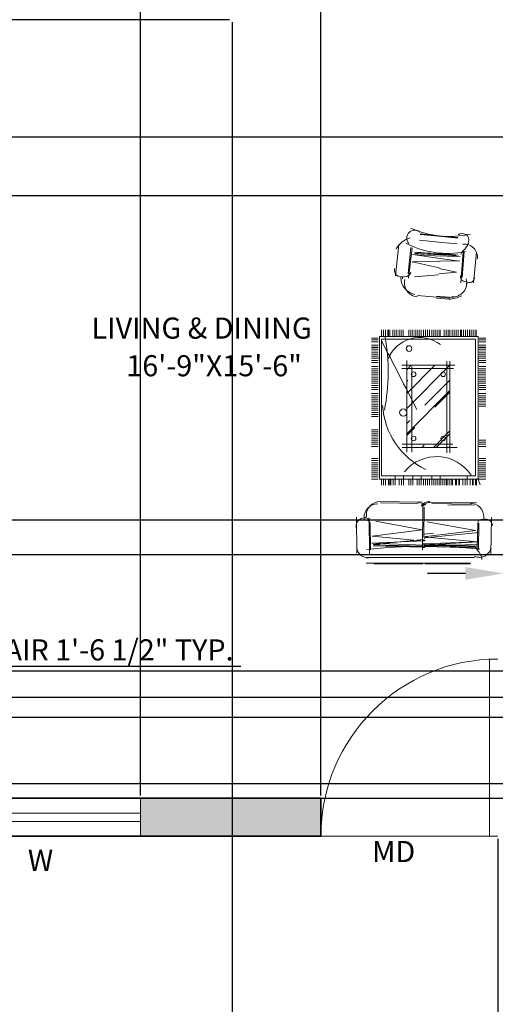
# Model space of a CAD drawing. Units: inches. Extents: x 2265 to 2807, y 1544 to 2401.
# Tile 7 of 9: x 2531 to 2643, y 1890 to 2124. Entities that reach past the tile are written whole.
import ezdxf

# ---------------------------------------------------------------- set-up
doc = ezdxf.new("R2010")
doc.units = ezdxf.units.IN
for name, color, linetype, lineweight in [('A-ANNO-DIMS', 2, 'Continuous', 18), ('A-ANNO-TEXT', 7, 'Continuous', 18), ('A-AREA-IDEN', 7, 'Continuous', 18), ('A-DOOR', 3, 'Continuous', 18), ('A-FURN-PATT', 161, 'Continuous', 13), ('A-GLAZ', 4, 'Continuous', 18), ('A-WALL', 7, 'Continuous', 35), ('A-WALL-PATT', 18, 'Continuous', 13), ('Furniture', 161, 'Continuous', 15)]:
    doc.layers.add(name, color=color, linetype=linetype, lineweight=lineweight)
doc.styles.add('ARIAL', font='times.ttf', dxfattribs={"height": 5})
doc.styles.get("Standard").update_dxf_attribs({"font": 'arial.ttf', "height": 5})
doc.dimstyles.new('ISO-25', dxfattribs={"dimtxt": 5, "dimasz": 9, "dimexe": 1.25, "dimexo": 0.625, "dimtad": 1, "dimlunit": 3, "dimtxsty": 'Standard', "dimcen": 2.5, "dimadec": 0, "dimazin": 0, "dimtfac": 1, "dimtmove": 0, "dimatfit": 3, "dimfxl": 1, "dimarcsym": 0})

# ---------------------------------------------------------------- blocks, each defined once
blk = doc.blocks.new('GLAZING-48IN')
for p, q in [((48, 9), (0, 9)), ((0, 5.5), (48, 5.5)), ((0, 5.5), (48, 5.5)), ((0, 3.5), (48, 3.5)), ((0, 0), (48, 0))]:
    blk.add_line(p, q)
blk = doc.blocks.new('DOOR-SWING-42IN')
for p, q in [((40, 41.95), (40, 0)), ((42, 0), (0, 0))]:
    blk.add_line(p, q)
blk.add_arc((42, 0), 42, 90, 180)
blk = doc.blocks.new('*D27')
at = {"layer": 'A-ANNO-DIMS', "color": 0, "lineweight": -2, "transparency": 16777216}
for p, q in [((2479.74, 1968.41), (2479.74, 1971.79)), ((2498.12, 1968.41), (2498.12, 1971.79)), ((2470.74, 1970.54), (2461.74, 1970.54)), ((2479.74, 1970.54), (2498.12, 1970.54)), ((2507.12, 1970.54), (2583.11, 1970.54))]:
    blk.add_line(p, q, dxfattribs=at)
at = {"layer": 'A-ANNO-DIMS', "color": 0, "lineweight": 100, "transparency": 16777216}
for points in [[(2470.74, 1972.04), (2470.74, 1969.04), (2479.74, 1970.54)], [(2507.12, 1972.04), (2507.12, 1969.04), (2498.12, 1970.54)]]:
    blk.add_solid(points, dxfattribs=at)
at = {"layer": 'Defpoints', "color": 0, "lineweight": 100, "transparency": 16777216}
for p in [(2498.12, 1970.54), (2479.74, 1967.79), (2498.12, 1967.79)]:
    blk.add_point(p, dxfattribs=at)
at = {"layer": 'A-ANNO-DIMS', "color": 0, "transparency": 16777216, "insert": (2549.62, 1973.75), "char_height": 5, "attachment_point": 5}
blk.add_mtext('CHAIR 1\'-6 1/2" TYP.', dxfattribs=at)
blk = doc.blocks.new('*D29')
at = {"layer": 'A-ANNO-DIMS', "color": 0, "lineweight": -2, "transparency": 16777216}
for p, q in [((2645.38, 1993.96), (2645.38, 1991.27)), ((2659.2, 1993.96), (2659.2, 1991.27)), ((2636.38, 1992.52), (2627.38, 1992.52)), ((2645.38, 1992.52), (2659.2, 1992.52)), ((2668.2, 1992.52), (2749.43, 1992.52))]:
    blk.add_line(p, q, dxfattribs=at)
at = {"layer": 'A-ANNO-DIMS', "color": 0, "lineweight": 100, "transparency": 16777216}
for points in [[(2636.38, 1994.02), (2636.38, 1991.02), (2645.38, 1992.52)], [(2668.2, 1994.02), (2668.2, 1991.02), (2659.2, 1992.52)]]:
    blk.add_solid(points, dxfattribs=at)
at = {"layer": 'Defpoints', "color": 0, "lineweight": 100, "transparency": 16777216}
for p in [(2645.38, 1994.59), (2659.2, 1994.59), (2659.2, 1992.52)]:
    blk.add_point(p, dxfattribs=at)
at = {"layer": 'A-ANNO-DIMS', "color": 0, "transparency": 16777216, "insert": (2713.31, 1995.65), "char_height": 5, "attachment_point": 5}
blk.add_mtext('END TABLE 1\'-2" TYP.', dxfattribs=at)
blk = doc.blocks.new('*D35')
at = {"layer": 'A-ANNO-DIMS', "color": 0, "lineweight": -2, "transparency": 16777216}
for p, q in [((2581.1, 2123.11), (2581.1, 1546.93)), ((2662.1, 2123.11), (2662.1, 1546.93)), ((2590.1, 1548.18), (2653.1, 1548.18))]:
    blk.add_line(p, q, dxfattribs=at)
at = {"layer": 'A-ANNO-DIMS', "color": 0, "lineweight": 100, "transparency": 16777216}
for points in [[(2590.1, 1549.68), (2590.1, 1546.68), (2581.1, 1548.18)], [(2653.1, 1549.68), (2653.1, 1546.68), (2662.1, 1548.18)]]:
    blk.add_solid(points, dxfattribs=at)
at = {"layer": 'Defpoints', "color": 0, "lineweight": 100, "transparency": 16777216}
for p in [(2581.1, 2123.73), (2662.1, 2123.73), (2662.1, 1548.18)]:
    blk.add_point(p, dxfattribs=at)
at = {"layer": 'A-ANNO-DIMS', "color": 0, "transparency": 16777216, "insert": (2621.6, 1551.36), "char_height": 5, "attachment_point": 5}
blk.add_mtext('6\'-9"', dxfattribs=at)
blk = doc.blocks.new('*D39')
at = {"layer": 'A-ANNO-DIMS', "color": 0, "lineweight": -2, "transparency": 16777216}
for p, q in [((2644.1, 1929.61), (2644.1, 1546.93)), ((2662.1, 1929.61), (2662.1, 1546.93)), ((2635.1, 1548.18), (2626.1, 1548.18)), ((2644.1, 1548.18), (2662.1, 1548.18)), ((2671.1, 1548.18), (2680.1, 1548.18))]:
    blk.add_line(p, q, dxfattribs=at)
at = {"layer": 'A-ANNO-DIMS', "color": 0, "lineweight": 100, "transparency": 16777216}
for points in [[(2635.1, 1549.68), (2635.1, 1546.68), (2644.1, 1548.18)], [(2671.1, 1549.68), (2671.1, 1546.68), (2662.1, 1548.18)]]:
    blk.add_solid(points, dxfattribs=at)
at = {"layer": 'Defpoints', "color": 0, "lineweight": 100, "transparency": 16777216}
for p in [(2644.1, 1930.23), (2662.1, 1930.23), (2662.1, 1548.18)]:
    blk.add_point(p, dxfattribs=at)
at = {"layer": 'A-ANNO-DIMS', "color": 0, "transparency": 16777216, "insert": (2653.1, 1551.36), "char_height": 5, "attachment_point": 5}
blk.add_mtext('1\'-6"', dxfattribs=at)
blk = doc.blocks.new('*D41')
at = {"layer": 'A-ANNO-DIMS', "color": 0, "lineweight": -2, "transparency": 16777216}
for p, q in [((2392.73, 2005.23), (2804.46, 2005.23)), ((2803.21, 1996.23), (2803.21, 1972.23)), ((2392.73, 1963.23), (2804.46, 1963.23))]:
    blk.add_line(p, q, dxfattribs=at)
at = {"layer": 'A-ANNO-DIMS', "color": 0, "lineweight": 100, "transparency": 16777216}
for points in [[(2801.71, 1996.23), (2804.71, 1996.23), (2803.21, 2005.23)], [(2801.71, 1972.23), (2804.71, 1972.23), (2803.21, 1963.23)]]:
    blk.add_solid(points, dxfattribs=at)
at = {"layer": 'Defpoints', "color": 0, "lineweight": 100, "transparency": 16777216}
for p in [(2392.1, 2005.23), (2392.1, 1963.23), (2803.21, 1963.23)]:
    blk.add_point(p, dxfattribs=at)
at = {"layer": 'A-ANNO-DIMS', "color": 0, "transparency": 16777216, "insert": (2800.03, 1984.23), "char_height": 5, "attachment_point": 5, "rotation": 90}
blk.add_mtext('3\'-6"', dxfattribs=at)
blk = doc.blocks.new('*D42')
at = {"layer": 'A-ANNO-DIMS', "color": 0, "lineweight": -2, "transparency": 16777216}
for p, q in [((2464.73, 1963.23), (2804.46, 1963.23)), ((2803.21, 1954.23), (2803.21, 1948.23)), ((2464.73, 1939.23), (2804.46, 1939.23))]:
    blk.add_line(p, q, dxfattribs=at)
at = {"layer": 'A-ANNO-DIMS', "color": 0, "lineweight": 100, "transparency": 16777216}
for points in [[(2801.71, 1954.23), (2804.71, 1954.23), (2803.21, 1963.23)], [(2801.71, 1948.23), (2804.71, 1948.23), (2803.21, 1939.23)]]:
    blk.add_solid(points, dxfattribs=at)
at = {"layer": 'Defpoints', "color": 0, "lineweight": 100, "transparency": 16777216}
for p in [(2464.1, 1963.23), (2464.1, 1939.23), (2803.21, 1939.23)]:
    blk.add_point(p, dxfattribs=at)
at = {"layer": 'A-ANNO-DIMS', "color": 0, "transparency": 16777216, "insert": (2800.03, 1951.23), "char_height": 5, "attachment_point": 5, "rotation": 90}
blk.add_mtext('2\'-0"', dxfattribs=at)
blk = doc.blocks.new('*D46')
at = {"layer": 'A-ANNO-DIMS', "color": 0, "lineweight": -2, "transparency": 16777216}
for p, q in [((2803.21, 2104.95), (2803.21, 2128.02)), ((2381.23, 2095.95), (2804.46, 2095.95)), ((2803.21, 2082.06), (2803.21, 2095.95)), ((2381.23, 2082.06), (2804.46, 2082.06)), ((2803.21, 2073.06), (2803.21, 2064.06))]:
    blk.add_line(p, q, dxfattribs=at)
at = {"layer": 'A-ANNO-DIMS', "color": 0, "lineweight": 100, "transparency": 16777216}
for points in [[(2801.71, 2104.95), (2804.71, 2104.95), (2803.21, 2095.95)], [(2801.71, 2073.06), (2804.71, 2073.06), (2803.21, 2082.06)]]:
    blk.add_solid(points, dxfattribs=at)
at = {"layer": 'Defpoints', "color": 0, "lineweight": 100, "transparency": 16777216}
for p in [(2380.61, 2095.95), (2803.21, 2095.95), (2380.61, 2082.06)]:
    blk.add_point(p, dxfattribs=at)
at = {"layer": 'A-ANNO-DIMS', "color": 0, "transparency": 16777216, "insert": (2800.07, 2120.99), "char_height": 5, "attachment_point": 5, "rotation": 90}
blk.add_mtext('1\'-2"', dxfattribs=at)
blk = doc.blocks.new('*D52')
at = {"layer": 'A-ANNO-DIMS', "color": 0, "lineweight": -2, "transparency": 16777216}
for p, q in [((2559.35, 1939.86), (2559.35, 2297.59)), ((2568.35, 2296.34), (2593.1, 2296.34)), ((2602.1, 1939.86), (2602.1, 2297.59))]:
    blk.add_line(p, q, dxfattribs=at)
at = {"layer": 'A-ANNO-DIMS', "color": 0, "lineweight": 100, "transparency": 16777216}
for points in [[(2568.35, 2297.84), (2568.35, 2294.84), (2559.35, 2296.34)], [(2593.1, 2297.84), (2593.1, 2294.84), (2602.1, 2296.34)]]:
    blk.add_solid(points, dxfattribs=at)
at = {"layer": 'Defpoints', "color": 0, "lineweight": 100, "transparency": 16777216}
for p in [(2602.1, 2296.34), (2559.35, 1939.23), (2602.1, 1939.23)]:
    blk.add_point(p, dxfattribs=at)
at = {"layer": 'A-ANNO-DIMS', "color": 0, "transparency": 16777216, "insert": (2580.73, 2299.52), "char_height": 5, "attachment_point": 5}
blk.add_mtext('3\'-7"', dxfattribs=at)
blk = doc.blocks.new('*D60')
at = {"layer": 'A-ANNO-DIMS', "color": 0, "lineweight": -2, "transparency": 16777216}
for p, q in [((2275.29, 2142.73), (2275.29, 2151.73)), ((2580.48, 2133.73), (2274.04, 2133.73)), ((2275.29, 2133.73), (2275.29, 2123.73)), ((2580.48, 2123.73), (2274.04, 2123.73)), ((2275.29, 2114.73), (2275.29, 2087.31))]:
    blk.add_line(p, q, dxfattribs=at)
at = {"layer": 'A-ANNO-DIMS', "color": 0, "lineweight": 100, "transparency": 16777216}
for points in [[(2273.79, 2142.73), (2276.79, 2142.73), (2275.29, 2133.73)], [(2273.79, 2114.73), (2276.79, 2114.73), (2275.29, 2123.73)]]:
    blk.add_solid(points, dxfattribs=at)
at = {"layer": 'Defpoints', "color": 0, "lineweight": 100, "transparency": 16777216}
for p in [(2581.1, 2133.73), (2275.29, 2123.73), (2581.1, 2123.73)]:
    blk.add_point(p, dxfattribs=at)
at = {"layer": 'A-ANNO-DIMS', "color": 0, "transparency": 16777216, "insert": (2272.11, 2096.52), "char_height": 5, "attachment_point": 5, "rotation": 90}
blk.add_mtext('0\'-10"', dxfattribs=at)
blk = doc.blocks.new('*D61')
at = {"layer": 'A-ANNO-DIMS', "color": 0, "lineweight": -2, "transparency": 16777216}
for p, q in [((2803.21, 1967.45), (2803.21, 1976.45)), ((2444.67, 1958.45), (2804.46, 1958.45)), ((2803.21, 1958.45), (2803.21, 1942.7)), ((2444.67, 1942.7), (2804.46, 1942.7)), ((2803.21, 1933.7), (2803.21, 1898.98))]:
    blk.add_line(p, q, dxfattribs=at)
at = {"layer": 'A-ANNO-DIMS', "color": 0, "lineweight": 100, "transparency": 16777216}
for points in [[(2801.71, 1967.45), (2804.71, 1967.45), (2803.21, 1958.45)], [(2801.71, 1933.7), (2804.71, 1933.7), (2803.21, 1942.7)]]:
    blk.add_solid(points, dxfattribs=at)
at = {"layer": 'Defpoints', "color": 0, "lineweight": 100, "transparency": 16777216}
for p in [(2444.05, 1958.45), (2444.05, 1942.7), (2803.21, 1942.7)]:
    blk.add_point(p, dxfattribs=at)
at = {"layer": 'A-ANNO-DIMS', "color": 0, "transparency": 16777216, "insert": (2800, 1911.84), "char_height": 5, "attachment_point": 5, "rotation": 90}
blk.add_mtext('1\'-3 1/2"', dxfattribs=at)
blk = doc.blocks.new('*D64')
at = {"layer": 'A-ANNO-DIMS', "color": 0, "lineweight": -2, "transparency": 16777216}
for p, q in [((2521.03, 1996.97), (2804.46, 1996.97)), ((2803.21, 1978.41), (2803.21, 1987.97)), ((2521.03, 1969.41), (2804.46, 1969.41))]:
    blk.add_line(p, q, dxfattribs=at)
at = {"layer": 'A-ANNO-DIMS', "color": 0, "lineweight": 100, "transparency": 16777216}
for points in [[(2801.71, 1987.97), (2804.71, 1987.97), (2803.21, 1996.97)], [(2801.71, 1978.41), (2804.71, 1978.41), (2803.21, 1969.41)]]:
    blk.add_solid(points, dxfattribs=at)
at = {"layer": 'Defpoints', "color": 0, "lineweight": 100, "transparency": 16777216}
for p in [(2520.4, 1996.97), (2803.21, 1996.97), (2520.4, 1969.41)]:
    blk.add_point(p, dxfattribs=at)
at = {"layer": 'A-ANNO-DIMS', "color": 0, "transparency": 16777216, "insert": (2800, 1983.19), "char_height": 5, "attachment_point": 5, "rotation": 90}
blk.add_mtext('2\'-3 1/2"', dxfattribs=at)

msp = doc.modelspace()

# ---------------------------------------------------------------- hatches: boundary and pattern name
at = {"layer": 'A-FURN-PATT'}
h = msp.add_hatch(dxfattribs=at)
h.set_pattern_fill('AR-RROOF', color=256, scale=0.266265, angle=585, style=0)
h.set_pattern_definition([(225, (3863.236, 2357.7255), (-5.7387, -15.3032), [101.44684, -13.52625, 33.8156, -6.76312]), (225, (3859.267, 2348.974), (11.14264, -1.57814), [20.28937, -2.23183, 40.57874, -5.07234]), (225, (3864.91, 2351.2695), (-21.663592, -28.071807), [54.10498, -9.46837, 27.05249, -6.76312])])
h.paths.add_polyline_path([(2622.465, 2022.355), (2632.719, 2022.355), (2632.719, 2041.841), (2622.465, 2041.841)])
at = {"layer": 'A-WALL-PATT'}
h = msp.add_hatch(color=256, dxfattribs=at)
h.dxf.hatch_style = 1
h.paths.add_polyline_path([(2602.101, 1939.233), (2559.351, 1939.233), (2559.351, 1930.233), (2602.101, 1930.233)])

# ---------------------------------------------------------------- linework, layer by layer
at = {"layer": 'A-GLAZ'}
msp.add_line((2559.351, 1930.233), (2559.351, 1939.233), dxfattribs=at)
at = {"layer": 'A-WALL'}
for p, q in [((2602.101, 1939.233), (2468.601, 1939.233)), ((2602.101, 1939.233), (2602.101, 1930.233)), ((2602.101, 1930.233), (2368.101, 1930.233))]:
    msp.add_line(p, q, dxfattribs=at)
at = {"layer": 'Furniture'}
for p, q in [((2625.638, 2072.819), (2630.883, 2072.324)), ((2625.652, 2072.969), (2630.897, 2072.474)), ((2630.883, 2072.324), (2634.557, 2071.977)), ((2630.897, 2072.474), (2634.571, 2072.127)), ((2619.772, 2063.047), (2620.583, 2070.456)), ((2622.77, 2063.613), (2623.459, 2069.781)), ((2622.875, 2062.461), (2623.723, 2069.661)), ((2625.511, 2071.467), (2630.756, 2070.972)), ((2630.756, 2070.972), (2634.43, 2070.625)), ((2630.397, 2067.172), (2623.848, 2068.074)), ((2623.848, 2068.074), (2630.449, 2067.722)), ((2630.453, 2067.769), (2635.095, 2067.522)), ((2635.281, 2061.372), (2635.805, 2068.741)), ((2635.608, 2062.621), (2636.086, 2068.809)), ((2639.033, 2068.684), (2638.324, 2061.402)), ((2630.325, 2066.416), (2623.791, 2066.374)), ((2623.791, 2066.374), (2630.186, 2064.946)), ((2635.021, 2066.564), (2630.336, 2066.534)), ((2634.941, 2066.496), (2630.392, 2067.123)), ((2621.534, 2062.871), (2621.467, 2062.288)), ((2622.041, 2062.787), (2621.758, 2062.82)), ((2630.029, 2063.284), (2624.329, 2062.775)), ((2634.294, 2063.879), (2630.05, 2063.5)), ((2630.173, 2064.799), (2634.294, 2063.879)), ((2621.985, 2062.173), (2621.942, 2061.587)), ((2621.985, 2062.173), (2621.942, 2061.587)), ((2636.169, 2061.674), (2636.454, 2061.653)), ((2636.683, 2061.661), (2636.64, 2061.076)), ((2629.531, 2058.002), (2625.026, 2058.35)), ((2632.71, 2057.777), (2629.532, 2058.022)), ((2633.538, 2057.935), (2629.553, 2058.243)), ((2632.498, 2057.501), (2629.505, 2057.731)), ((2616.007, 2048.698), (2639.384, 2048.698)), ((2616.007, 2014.891), (2616.007, 2048.698)), ((2616.486, 2048.705), (2616.486, 2050.258)), ((2616.979, 2048.705), (2616.979, 2050.258)), ((2617.472, 2048.705), (2617.472, 2050.258)), ((2617.965, 2048.705), (2617.965, 2050.258)), ((2618.153, 2048.705), (2618.153, 2050.258)), ((2618.459, 2048.705), (2618.459, 2050.258)), ((2619.159, 2048.705), (2619.159, 2050.258)), ((2619.652, 2048.705), (2619.652, 2050.258)), ((2620.145, 2048.705), (2620.145, 2050.258)), ((2620.639, 2048.705), (2620.639, 2050.258)), ((2621.132, 2048.705), (2621.132, 2050.258)), ((2621.625, 2048.705), (2621.625, 2050.258)), ((2622.955, 2048.705), (2622.955, 2050.258)), ((2623.449, 2048.705), (2623.449, 2050.258)), ((2623.942, 2048.705), (2623.942, 2050.258)), ((2624.435, 2048.705), (2624.435, 2050.258)), ((2624.928, 2048.705), (2624.928, 2050.258)), ((2625.422, 2048.705), (2625.422, 2050.258)), ((2625.915, 2048.705), (2625.915, 2050.258)), ((2626.408, 2048.705), (2626.408, 2050.258)), ((2626.901, 2048.705), (2626.901, 2050.258)), ((2627.395, 2048.705), (2627.395, 2050.258)), ((2627.888, 2048.705), (2627.888, 2050.258)), ((2628.381, 2048.705), (2628.381, 2050.258)), ((2628.874, 2048.705), (2628.874, 2050.258)), ((2629.368, 2048.705), (2629.368, 2050.258)), ((2629.85, 2048.705), (2629.85, 2050.258)), ((2629.861, 2048.705), (2629.861, 2050.258)), ((2630.344, 2048.705), (2630.344, 2050.258)), ((2630.354, 2048.705), (2630.354, 2050.258)), ((2631.339, 2048.705), (2631.339, 2050.258)), ((2631.832, 2048.705), (2631.832, 2050.258)), ((2632.326, 2048.705), (2632.326, 2050.258)), ((2632.72, 2048.705), (2632.72, 2050.258)), ((2633.213, 2048.705), (2633.213, 2050.258)), ((2633.706, 2048.705), (2633.706, 2050.258)), ((2634.199, 2048.705), (2634.199, 2050.258)), ((2634.682, 2048.705), (2634.682, 2050.258)), ((2634.693, 2048.705), (2634.693, 2050.258)), ((2635.176, 2048.705), (2635.176, 2050.258)), ((2635.186, 2048.705), (2635.186, 2050.258)), ((2635.422, 2048.705), (2635.422, 2050.258)), ((2635.915, 2048.705), (2635.915, 2050.258)), ((2636.408, 2048.705), (2636.408, 2050.258)), ((2636.891, 2048.705), (2636.891, 2050.258)), ((2636.902, 2048.705), (2636.902, 2050.258)), ((2637.384, 2048.705), (2637.384, 2050.258)), ((2637.395, 2048.705), (2637.395, 2050.258)), ((2637.906, 2048.705), (2637.906, 2050.258)), ((2638.388, 2048.705), (2638.388, 2050.258)), ((2638.399, 2048.705), (2638.399, 2050.258)), ((2638.882, 2048.705), (2638.882, 2050.258)), ((2638.892, 2048.705), (2638.892, 2050.258)), ((2639.384, 2048.698), (2639.384, 2014.891)), ((2615.665, 2048.254), (2614.112, 2048.254)), ((2615.665, 2047.854), (2614.112, 2047.854)), ((2615.665, 2047.361), (2614.112, 2047.361)), ((2615.665, 2046.622), (2614.112, 2046.622)), ((2616.496, 2048.008), (2638.807, 2048.008)), ((2616.496, 2048.008), (2616.496, 2015.679)), ((2638.807, 2015.679), (2638.807, 2048.008)), ((2639.638, 2048.254), (2641.191, 2048.254)), ((2639.638, 2047.854), (2641.191, 2047.854)), ((2639.638, 2047.361), (2641.191, 2047.361)), ((2639.638, 2046.622), (2641.191, 2046.622)), ((2615.665, 2046.128), (2614.112, 2046.128)), ((2615.665, 2045.966), (2614.112, 2045.966)), ((2615.665, 2045.472), (2614.112, 2045.472)), ((2615.665, 2044.979), (2614.112, 2044.979)), ((2615.665, 2044.486), (2614.112, 2044.486)), ((2615.665, 2043.992), (2614.112, 2043.992)), ((2639.638, 2046.128), (2641.191, 2046.128)), ((2639.638, 2045.966), (2641.191, 2045.966)), ((2639.638, 2045.472), (2641.191, 2045.472)), ((2639.638, 2044.979), (2641.191, 2044.979)), ((2639.638, 2044.486), (2641.191, 2044.486)), ((2639.638, 2043.992), (2641.191, 2043.992)), ((2615.918, 2043.499), (2614.112, 2043.499)), ((2615.665, 2043.006), (2614.112, 2043.006)), ((2615.665, 2042.513), (2614.112, 2042.513)), ((2621.329, 2041.841), (2633.837, 2041.841)), ((2622.465, 2021.233), (2622.465, 2042.951)), ((2623.678, 2021.233), (2623.678, 2041.58)), ((2631.963, 2042.798), (2631.963, 2021.08)), ((2632.719, 2042.798), (2632.719, 2021.08)), ((2639.384, 2043.499), (2641.191, 2043.499)), ((2639.638, 2043.006), (2641.191, 2043.006)), ((2639.638, 2042.513), (2641.191, 2042.513)), ((2615.665, 2041.526), (2614.112, 2041.526)), ((2615.665, 2041.033), (2614.112, 2041.033)), ((2615.665, 2040.54), (2614.112, 2040.54)), ((2615.665, 2040.046), (2614.112, 2040.046)), ((2615.665, 2039.553), (2614.112, 2039.553)), ((2621.329, 2041.085), (2633.568, 2041.085)), ((2639.638, 2041.526), (2641.191, 2041.526)), ((2639.638, 2041.033), (2641.191, 2041.033)), ((2639.638, 2040.54), (2641.191, 2040.54)), ((2639.638, 2040.046), (2641.191, 2040.046)), ((2639.638, 2039.553), (2641.191, 2039.553)), ((2615.665, 2039.06), (2614.112, 2039.06)), ((2615.665, 2038.567), (2614.112, 2038.567)), ((2615.665, 2038.073), (2614.112, 2038.073)), ((2615.665, 2037.58), (2614.112, 2037.58)), ((2615.665, 2037.087), (2614.112, 2037.087)), ((2639.638, 2039.06), (2641.191, 2039.06)), ((2639.638, 2038.567), (2641.191, 2038.567)), ((2639.638, 2038.073), (2641.191, 2038.073)), ((2639.638, 2037.58), (2641.191, 2037.58)), ((2639.638, 2037.087), (2641.191, 2037.087)), ((2615.665, 2036.594), (2614.112, 2036.594)), ((2615.665, 2036.1), (2614.112, 2036.1)), ((2615.665, 2035.114), (2614.112, 2035.114)), ((2615.665, 2034.621), (2614.112, 2034.621)), ((2639.638, 2036.594), (2641.191, 2036.594)), ((2639.638, 2036.1), (2641.191, 2036.1)), ((2639.638, 2035.114), (2641.191, 2035.114)), ((2639.638, 2034.621), (2641.191, 2034.621)), ((2615.665, 2034.127), (2614.112, 2034.127)), ((2615.665, 2033.634), (2614.112, 2033.634)), ((2615.665, 2033.141), (2614.112, 2033.141)), ((2615.665, 2032.648), (2614.112, 2032.648)), ((2639.638, 2034.127), (2641.191, 2034.127)), ((2639.638, 2033.634), (2641.191, 2033.634)), ((2639.638, 2033.141), (2641.191, 2033.141)), ((2639.638, 2032.648), (2641.191, 2032.648)), ((2615.665, 2032.154), (2614.112, 2032.154)), ((2615.665, 2031.661), (2614.112, 2031.661)), ((2615.665, 2031.168), (2614.112, 2031.168)), ((2615.665, 2030.675), (2614.112, 2030.675)), ((2615.665, 2030.181), (2614.112, 2030.181)), ((2639.638, 2032.154), (2641.191, 2032.154)), ((2615.665, 2029.688), (2614.112, 2029.688)), ((2615.665, 2026.563), (2614.112, 2026.563)), ((2615.665, 2026.07), (2614.112, 2026.07)), ((2615.665, 2025.576), (2614.112, 2025.576)), ((2615.665, 2025.083), (2614.112, 2025.083)), ((2615.665, 2024.59), (2614.112, 2024.59)), ((2615.665, 2024.097), (2614.112, 2024.097)), ((2615.665, 2023.603), (2614.112, 2023.603)), ((2615.665, 2023.11), (2614.112, 2023.11)), ((2633.416, 2023.112), (2621.399, 2023.112)), ((2639.638, 2024.097), (2641.191, 2024.097)), ((2639.638, 2023.603), (2641.191, 2023.603)), ((2639.638, 2023.11), (2641.191, 2023.11)), ((2615.665, 2022.617), (2614.112, 2022.617)), ((2634.401, 2022.355), (2621.399, 2022.355)), ((2639.638, 2022.617), (2641.191, 2022.617)), ((2615.665, 2019.747), (2614.112, 2019.747)), ((2615.665, 2019.254), (2614.112, 2019.254)), ((2615.665, 2018.761), (2614.112, 2018.761)), ((2615.665, 2018.268), (2614.112, 2018.268)), ((2639.638, 2019.747), (2641.191, 2019.747)), ((2639.638, 2019.254), (2641.191, 2019.254)), ((2639.638, 2018.761), (2641.191, 2018.761)), ((2639.638, 2018.268), (2641.191, 2018.268)), ((2615.665, 2017.774), (2614.112, 2017.774)), ((2615.665, 2017.281), (2614.112, 2017.281)), ((2615.665, 2016.861), (2614.112, 2016.861)), ((2615.665, 2016.368), (2614.112, 2016.368)), ((2639.638, 2017.774), (2641.191, 2017.774)), ((2639.638, 2017.281), (2641.191, 2017.281)), ((2639.638, 2016.861), (2641.191, 2016.861)), ((2639.638, 2016.368), (2641.191, 2016.368)), ((2615.665, 2015.874), (2614.112, 2015.874)), ((2615.665, 2015.381), (2614.112, 2015.381)), ((2615.665, 2014.888), (2614.112, 2014.888)), ((2640.414, 2014.888), (2616.007, 2014.891)), ((2616.486, 2014.968), (2616.486, 2013.415)), ((2616.496, 2015.679), (2638.807, 2015.679)), ((2616.979, 2014.968), (2616.979, 2013.415)), ((2617.472, 2014.968), (2617.472, 2013.415)), ((2618.153, 2014.968), (2618.153, 2013.415)), ((2618.459, 2014.968), (2618.459, 2013.415)), ((2618.737, 2014.968), (2618.737, 2013.415)), ((2619.23, 2014.968), (2619.23, 2013.415)), ((2619.723, 2015.679), (2619.723, 2013.415)), ((2620.71, 2014.968), (2620.71, 2013.415)), ((2621.203, 2014.968), (2621.203, 2013.415)), ((2621.696, 2015.679), (2621.696, 2013.415)), ((2622.955, 2014.968), (2622.955, 2013.415)), ((2623.449, 2014.968), (2623.449, 2013.415)), ((2623.942, 2015.679), (2623.942, 2013.415)), ((2624.928, 2014.968), (2624.928, 2013.415)), ((2625.422, 2014.968), (2625.422, 2013.415)), ((2625.915, 2015.679), (2625.915, 2013.415)), ((2626.408, 2014.968), (2626.408, 2013.415)), ((2626.901, 2014.968), (2626.901, 2013.415)), ((2627.395, 2014.968), (2627.395, 2013.415)), ((2627.888, 2014.968), (2627.888, 2013.415)), ((2628.381, 2015.679), (2628.381, 2013.415)), ((2628.874, 2014.968), (2628.874, 2013.415)), ((2629.368, 2014.968), (2629.368, 2013.415)), ((2629.85, 2014.968), (2629.85, 2013.415)), ((2629.861, 2014.968), (2629.861, 2013.415)), ((2630.344, 2014.968), (2630.344, 2013.415)), ((2630.354, 2015.679), (2630.354, 2013.415)), ((2630.837, 2014.968), (2630.837, 2013.415)), ((2630.847, 2014.968), (2630.847, 2013.415)), ((2631.33, 2014.968), (2631.33, 2013.415)), ((2631.341, 2014.968), (2631.341, 2013.415)), ((2631.824, 2014.968), (2631.824, 2013.415)), ((2631.834, 2014.968), (2631.834, 2013.415)), ((2632.026, 2014.968), (2632.026, 2013.415)), ((2632.519, 2014.968), (2632.519, 2013.415)), ((2633.013, 2014.968), (2633.013, 2013.415)), ((2633.303, 2014.968), (2633.303, 2013.415)), ((2633.999, 2014.968), (2633.999, 2013.415)), ((2634.29, 2014.968), (2634.29, 2013.415)), ((2634.783, 2014.968), (2634.783, 2013.415)), ((2634.986, 2014.968), (2634.986, 2013.415)), ((2635.804, 2014.968), (2635.804, 2013.415)), ((2636.297, 2014.968), (2636.297, 2013.415)), ((2636.791, 2015.679), (2636.791, 2013.415)), ((2637.541, 2014.968), (2637.541, 2013.415)), ((2638.034, 2014.968), (2638.034, 2013.415)), ((2638.237, 2014.968), (2638.237, 2013.415)), ((2638.73, 2014.968), (2638.73, 2013.415)), ((2639.021, 2014.968), (2639.021, 2013.415)), ((2639.33, 2015.052), (2639.851, 2013.491)), ((2639.638, 2015.874), (2641.191, 2015.874)), ((2639.638, 2015.381), (2641.191, 2015.381)), ((2639.638, 2014.888), (2641.191, 2014.888)), ((2626.131, 2009.399), (2615.524, 2009.563)), ((2625.144, 2009.105), (2616.268, 2009.257)), ((2626.304, 2009.04), (2626.202, 1998.118)), ((2639.03, 2009.226), (2627.653, 2009.391)), ((2637.727, 2008.932), (2628.397, 2009.084)), ((2626.576, 2008.232), (2626.514, 2001.243)), ((2638.537, 2008.696), (2632.239, 2008.796)), ((2610.675, 1997.287), (2610.566, 2005.873)), ((2612.366, 2005.083), (2612.354, 2005.67)), ((2612.879, 2005.119), (2612.594, 2005.113)), ((2612.881, 2005.736), (2612.893, 2006.323)), ((2612.881, 2005.736), (2612.893, 2006.323)), ((2613.527, 2005.67), (2613.633, 1997.061)), ((2613.78, 2004.255), (2613.907, 1998.118)), ((2626.147, 2002.881), (2615.158, 2004.916)), ((2638.73, 2002.708), (2627.287, 2004.743)), ((2639.32, 2004.419), (2639.193, 1998.282)), ((2639.573, 2004.393), (2639.467, 1998.188)), ((2640.221, 2005.283), (2640.506, 2005.278)), ((2640.733, 2005.247), (2640.745, 2005.834)), ((2642.533, 2005.802), (2642.425, 1997.113)), ((2614.284, 2001.384), (2626.147, 2002.881)), ((2626.413, 2001.211), (2638.73, 2002.708)), ((2626.661, 2001.838), (2628.826, 2002.055)), ((2626.758, 2000.983), (2639.536, 2002.219)), ((2626.545, 2000.214), (2614.181, 1999.686)), ((2614.181, 1999.686), (2626.601, 1999.178)), ((2626.618, 2000.139), (2614.284, 2001.384)), ((2614.472, 1999.386), (2626.428, 2000.586)), ((2626.75, 2000.378), (2626.278, 2000.358)), ((2626.822, 2000.303), (2626.278, 2000.358)), ((2639.129, 2000.041), (2626.31, 1999.514)), ((2639.201, 1999.966), (2626.413, 2001.211)), ((2626.6, 1999.213), (2639.129, 2000.041)), ((2626.661, 2000.753), (2626.758, 2000.762)), ((2639.185, 1999.006), (2639.201, 1999.966)), ((2626.287, 1998.68), (2626.661, 1998.68)), ((2626.31, 1999.514), (2639.185, 1999.006)), ((2626.661, 1999.348), (2626.806, 1999.342)), ((2626.661, 1998.68), (2626.758, 1998.68)), ((2612.833, 1994.958), (2626.287, 1994.958)), ((2612.924, 1996.316), (2626.287, 1996.316)), ((2626.287, 1996.316), (2626.661, 1996.316)), ((2626.287, 1994.958), (2626.661, 1994.958)), ((2626.661, 1996.316), (2626.758, 1996.316)), ((2626.661, 1994.958), (2626.758, 1994.958)), ((2626.758, 1996.316), (2638.55, 1996.316)), ((2626.758, 1994.958), (2637.583, 1994.958)), ((2614.695, 1994.807), (2626.287, 1994.807)), ((2626.758, 1994.807), (2637.583, 1994.807))]:
    msp.add_line(p, q, dxfattribs=at)
for centre, radius in [((2623.018, 2045.808), 0.665), ((2624.091, 2039.709), 0.54), ((2631.093, 2039.709), 0.54), ((2621.646, 2030.633), 0.861), ((2624.091, 2024.487), 0.54), ((2631.093, 2024.487), 0.54)]:
    msp.add_circle(centre, radius, dxfattribs=at)
for centre, radius, start, end in [((2632.569, 2094.612), 22.255, 245.53485, 283.0012), ((2624.711, 2066.738), 5.462, 105.05578, 150.33896), ((2624.343, 2072.002), 1.866, 46.59186, 222.74892), ((2635.615, 2071.517), 1.562, 344.59083, 129.17962), ((2631.996, 2089.109), 20.761, 241.93975, 282.11129), ((2636.138, 2067.433), 3.109, 352.65151, 96.80505), ((2575.055, 1249.914), 820.195, 86.124113, 86.559193), ((2615.044, 1816.936), 251.571, 86.48264, 87.87414), ((2613.877, 1817.046), 251.571, 85.37492, 86.21559), ((2573.889, 1250.024), 820.195, 85.74411, 86.042215), ((2600.42, 1818.537), 251.571, 81.87138, 81.93334), ((2621.188, 2064.415), 1.644, 168.01008, 285.81549), ((2621.958, 2064.309), 1.524, 273.1193, 342.10763), ((2636.387, 2062.857), 1.203, 169.02937, 259.59614), ((2625.189, 2062.719), 4.164, 182.69859, 258.54147), ((2625.227, 2061.346), 3.294, 175.79044, 265.79044), ((2633.324, 2061.411), 3.385, 266.425, 16.29431), ((2637.284, 2062.742), 1.306, 237.19555, 350.98549), ((2632.5, 2063.551), 6.018, 269.80149, 299.57333), ((1620.861, 1526.592), 1123.727, 26.692308, 27.623754), ((2569.461, 2040.33), 48.599, 349.17618, 9.73278), ((2625.526, 2040.446), 7.984, 51.9297, 160.04437), ((2634.639, 2033.37), 17.919, 183.34207, 244.81365), ((2629.542, 2010.389), 9.814, 33.37904, 140.51955), ((2615.648, 2005.738), 3.294, 91.18551, 181.18551), ((2616.186, 2006.255), 3.294, 88.81449, 178.81449), ((2624.868, 2006.075), 3.294, 53.48629, 88.81449), ((2627.609, 2007.609), 1.937, 81.24001, 153.3044), ((2624.84, 2006.24), 3.294, 53.48629, 61.16899), ((2625.023, 2006.24), 3.294, 53.48629, 61.16899), ((2628.315, 2006.082), 3.294, 88.81449, 118.20381), ((2637.452, 2005.903), 3.294, 358.81449, 88.81449), ((2628.1, 2005.903), 3.294, 120.50473, 128.40827), ((2628.284, 2005.903), 3.294, 120.50473, 128.40827), ((2612.456, 2003.68), 1.989, 46.00951, 198.15377), ((2612.897, 2004.237), 0.883, 1.18551, 91.18551), ((2640.202, 2004.401), 0.883, 88.81449, 178.81449), ((2641.203, 2003.746), 1.633, 5.65087, 110.59754), ((2613.327, 1998.882), 2.682, 171.46598, 272.13669), ((2626.754, 1877.977), 120.961, 83.80092, 96.53286), ((2642.53, 2818.81), 820.195, 268.045734, 268.860817), ((2629.028, 2250.54), 251.571, 266.73078, 269.3226), ((2627.064, 2250.54), 251.571, 269.82306, 269.90832), ((2629.233, 2250.704), 251.571, 269.41437, 269.43644), ((2655.749, 2883.805), 885.363, 268.119045, 268.903557), ((2627.046, 2269.68), 270.547, 269.93913, 272.63593), ((2648.706, 2584.514), 585.718, 267.857629, 269.021636), ((2639.728, 1999.022), 2.698, 242.8729, 358.81449)]:
    msp.add_arc(centre, radius, start, end, dxfattribs=at)
for points in [[(2637.12, 2071.102), (2637.028, 2069.905), (2635.612, 2068.895), (2635.263, 2068.19)], [(2640.281, 1995.807), (2640.301, 1997.008), (2638.987, 1998.147), (2638.705, 1998.882)]]:
    msp.add_open_spline(points, degree=3, dxfattribs=at)

# ---------------------------------------------------------------- block references
at = {"layer": 'A-DOOR'}
msp.add_blockref('DOOR-SWING-42IN', (2602.101, 1930.233), dxfattribs=at)
at = {"layer": 'A-GLAZ'}
msp.add_blockref('GLAZING-48IN', (2511.351, 1930.233), dxfattribs=at)

# ---------------------------------------------------------------- texts
at = {"layer": 'A-ANNO-TEXT', "style": 'ARIAL'}
for s, p in [('MD', (2614.254, 1924.115)), ('W', (2532.667, 1922.033))]:
    msp.add_text(s, height=5, dxfattribs=at).set_placement(p)
at = {"layer": 'A-AREA-IDEN', "style": 'ARIAL'}
for s, p in [('LIVING & DINING ', (2547.764, 2048.154)), (' 16\'-9"X15\'-6"', (2554.466, 2039.232))]:
    msp.add_text(s, height=5, dxfattribs=at).set_placement(p)

# ---------------------------------------------------------------- dimensions: what is measured, and where the dimension line sits
at = {"layer": 'A-ANNO-DIMS'}
for base, p1, p2, picture, middle in [((2602.101182, 2296.343269), (2559.351182, 1939.233269), (2602.101182, 1939.233269), '*D52', (2580.726182, 2299.522839259)), ((2662.101, 1548.185), (2581.101, 2123.733), (2662.101, 2123.733), '*D35', (2621.601, 1551.363)), ((2662.101, 1548.185), (2644.101, 1930.233), (2662.101, 1930.233), '*D39', (2653.101, 1551.363))]:
    dim = msp.add_linear_dim(base=base, p1=p1, p2=p2, dimstyle='ISO-25', override={"dimdec": 1, "dimlfac": 1, "dimrnd": 0, "dimzin": 1, "dimdsep": 46, "dimlunit": 4, "dimfrac": 2}, dxfattribs=at)
    dim.commit()
    dim.dimension.update_dxf_attribs({"geometry": picture, "text_midpoint": middle})
for base, p1, p2, picture, middle in [((2275.289, 2123.733), (2581.101, 2133.733), (2581.101, 2123.733), '*D60', (2272.111, 2096.52)), ((2803.21, 2095.951), (2380.607, 2082.055), (2380.607, 2095.951), '*D46', (2800.075, 2120.986)), ((2803.21, 1963.233), (2392.101, 2005.233), (2392.101, 1963.233), '*D41', (2800.03, 1984.233)), ((2803.21, 1996.968), (2520.405, 1969.409), (2520.405, 1996.968), '*D64', (2799.998, 1983.188)), ((2803.21, 1942.704), (2444.049, 1958.452), (2444.049, 1942.704), '*D61', (2799.998, 1911.843)), ((2803.21, 1939.233), (2464.101, 1963.233), (2464.101, 1939.233), '*D42', (2800.032, 1951.233))]:
    dim = msp.add_linear_dim(base=base, p1=p1, p2=p2, angle=90, dimstyle='ISO-25', override={"dimdec": 1, "dimlfac": 1, "dimrnd": 0, "dimzin": 1, "dimdsep": 46, "dimlunit": 4, "dimfrac": 2}, dxfattribs=at)
    dim.commit()
    dim.dimension.update_dxf_attribs({"geometry": picture, "text_midpoint": middle})
for base, p1, p2, text, picture, middle in [((2659.204, 1992.516), (2645.379, 1994.59), (2659.204, 1994.59), 'END TABLE <> TYP.', '*D29', (2713.315, 1995.653)), ((2498.119, 1970.542), (2479.739, 1967.785), (2498.119, 1967.785), 'CHAIR <> TYP.', '*D27', (2549.616, 1973.753))]:
    dim = msp.add_linear_dim(base=base, p1=p1, p2=p2, text=text, dimstyle='ISO-25', override={"dimdec": 1, "dimlfac": 1, "dimrnd": 0, "dimzin": 1, "dimdsep": 46, "dimlunit": 4, "dimfrac": 2}, dxfattribs=at)
    dim.commit()
    dim.dimension.update_dxf_attribs({"geometry": picture, "text_midpoint": middle})

doc.saveas('drawing.dxf')
